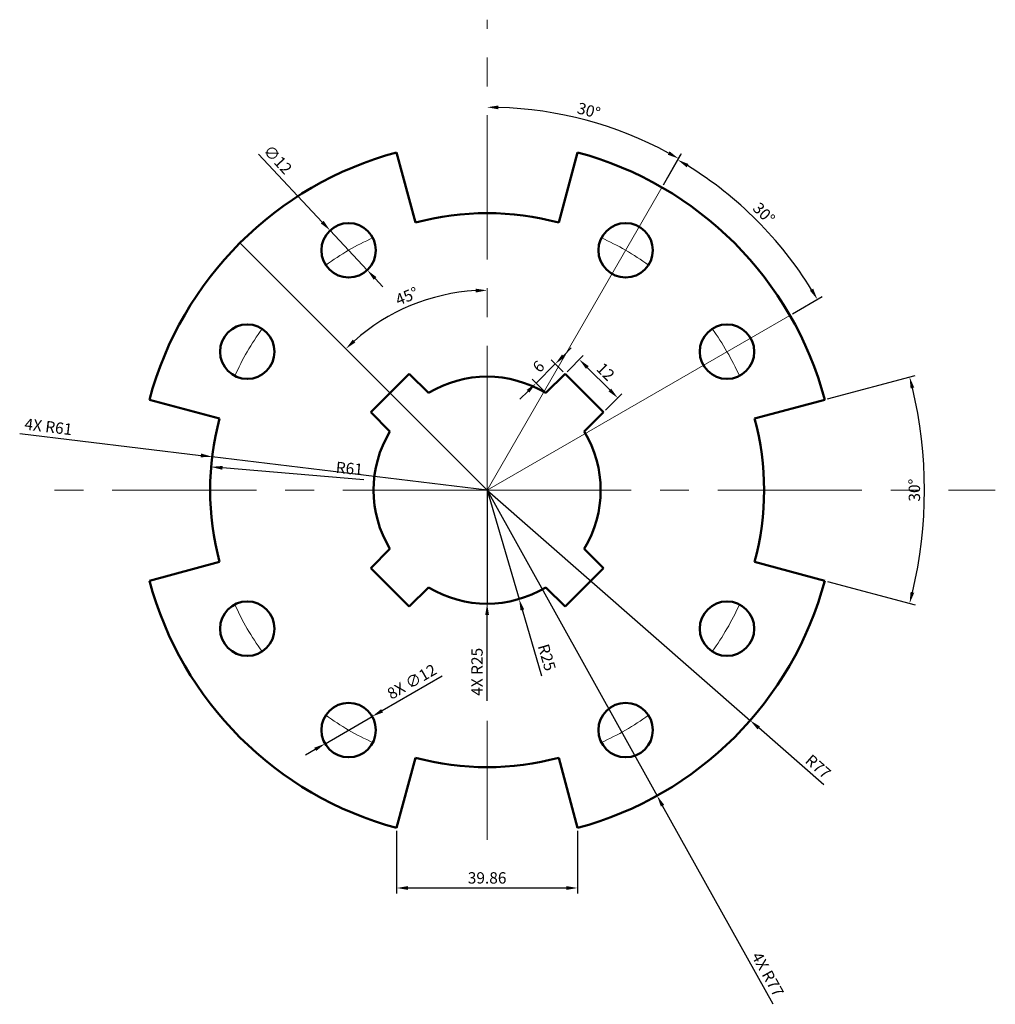
# Model space of a CAD drawing. Units: millimetres. Extents: x -38 to 176, y -46 to 171.
import ezdxf

# ---------------------------------------------------------------- set-up
doc = ezdxf.new("R2010")
doc.units = ezdxf.units.MM
doc.linetypes.add('CENTER', pattern=[50.8, 31.75, -6.35, 6.35, -6.35])
for name, color, linetype, lineweight in [('M-CNTR', 4, 'CENTER', 18), ('M-CONS', 8, 'Continuous', 13), ('M-DIMS', 2, 'Continuous', 25), ('M-OUTL', 7, 'Continuous', 50)]:
    doc.layers.add(name, color=color, linetype=linetype, lineweight=lineweight)
doc.styles.get("Standard").update_dxf_attribs({"font": 'arial.ttf'})
doc.dimstyles.new('ISO-25', dxfattribs={"dimtxt": 2.5, "dimasz": 2.5, "dimexe": 1.25, "dimexo": 0.625, "dimtad": 1, "dimtxsty": 'Standard', "dimcen": 2.5, "dimadec": 0, "dimazin": 0, "dimtfac": 1, "dimtmove": 0, "dimatfit": 3, "dimfxl": 1, "dimarcsym": 0})

# ---------------------------------------------------------------- blocks, each defined once
blk = doc.blocks.new('*U1')
for p, q in [((-6.36, 2.12), (-2.12, 6.36)), ((-2.12, 6.36), (6.36, -2.12)), ((2.12, -6.36), (6.36, -2.12))]:
    blk.add_line(p, q)
blk = doc.blocks.new('*U2')
at = {"layer": 'M-OUTL', "color": 0, "linetype": 'ByBlock', "lineweight": -2, "transparency": 16777216}
for p, rotation in [((45.29, 86.23), 90.00000000000003), ((45.29, 47.67), 180), ((83.86, 47.67), 270)]:
    blk.add_blockref('*U1', p, dxfattribs=dict(at, rotation=rotation))
blk.add_blockref('*U1', (83.86, 86.23), dxfattribs=at)
blk = doc.blocks.new('*D3')
at = {"layer": 'Defpoints', "color": 0, "transparency": 16777216}
for p in [(81.74, 92.59), (93.36, 87.25), (90.22, 84.11)]:
    blk.add_point(p, dxfattribs=at)
at = {"layer": 'M-DIMS', "color": 0, "lineweight": -2, "transparency": 16777216}
for p, q in [((82.18, 93.04), (85.76, 96.62)), ((86.64, 93.97), (91.59, 89.02)), ((90.66, 84.55), (94.24, 88.13))]:
    blk.add_line(p, q, dxfattribs=at)
at = {"layer": 'M-DIMS', "color": 0, "transparency": 16777216}
for points in [[(86.94, 94.26), (86.35, 93.67), (84.87, 95.73)], [(91.89, 89.31), (91.3, 88.72), (93.36, 87.25)]]:
    blk.add_solid(points, dxfattribs=at)
at = {"layer": 'M-DIMS', "color": 0, "transparency": 16777216, "insert": (90.45, 92.82), "char_height": 2.5, "attachment_point": 5, "rotation": 315}
blk.add_mtext('12', dxfattribs=at)
blk = doc.blocks.new('*D4')
at = {"layer": 'Defpoints', "color": 0, "transparency": 16777216}
for p in [(79.59, 94.74), (81.74, 92.59), (77.49, 88.35)]:
    blk.add_point(p, dxfattribs=at)
at = {"layer": 'M-DIMS', "color": 0, "lineweight": -2, "transparency": 16777216}
for p, q in [((81.36, 96.51), (83.12, 98.28)), ((81.29, 93.04), (78.7, 95.63)), ((75.35, 90.5), (79.59, 94.74)), ((77.05, 88.79), (74.46, 91.38)), ((73.58, 88.73), (71.81, 86.96))]:
    blk.add_line(p, q, dxfattribs=at)
at = {"layer": 'M-DIMS', "color": 0, "transparency": 16777216}
for points in [[(81.06, 96.8), (81.65, 96.21), (79.59, 94.74)], [(73.28, 89.03), (73.87, 88.44), (75.35, 90.5)]]:
    blk.add_solid(points, dxfattribs=at)
at = {"layer": 'M-DIMS', "color": 0, "transparency": 16777216, "insert": (76.12, 93.96), "char_height": 2.5, "attachment_point": 5, "rotation": 45}
blk.add_mtext('6', dxfattribs=at)
blk = doc.blocks.new('*D5')
at = {"layer": 'Defpoints', "color": 0, "transparency": 16777216}
for p in [(64.57, 170.55), (10.13, 121.39), (53.18, 109.46), (64.57, 66.95), (64.57, 66.95)]:
    blk.add_point(p, dxfattribs=at)
at = {"layer": 'M-DIMS', "color": 0, "lineweight": -2, "transparency": 16777216}
blk.add_arc((64.57, 66.95), 44.01, 93.255, 131.745, dxfattribs=at)
at = {"layer": 'M-DIMS', "color": 0, "transparency": 16777216}
for points in [[(62.06, 111.31), (62.09, 110.47), (64.57, 110.96)], [(35.56, 99.48), (34.98, 100.09), (33.45, 98.07)]]:
    blk.add_solid(points, dxfattribs=at)
at = {"layer": 'M-DIMS', "color": 0, "transparency": 16777216, "insert": (47.01, 109.36), "char_height": 2.5, "attachment_point": 5, "rotation": 22.5}
blk.add_mtext('45°', dxfattribs=at)
blk = doc.blocks.new('*D6')
at = {"layer": 'Defpoints', "color": 0, "transparency": 16777216}
for p in [(138.95, 86.88), (123.5, 82.74), (160.54, 58.55), (123.5, 51.16), (138.95, 47.02)]:
    blk.add_point(p, dxfattribs=at)
at = {"layer": 'M-DIMS', "color": 0, "lineweight": -2, "transparency": 16777216}
for p, q in [((139.55, 87.04), (158.83, 92.2)), ((139.55, 46.86), (158.83, 41.69))]:
    blk.add_line(p, q, dxfattribs=at)
blk.add_arc((64.57, 66.95), 96.33, 346.487, 13.513, dxfattribs=at)
at = {"layer": 'M-DIMS', "color": 0, "transparency": 16777216}
for points in [[(157.84, 89.35), (158.64, 89.56), (157.62, 91.88)], [(158.64, 44.34), (157.84, 44.54), (157.62, 42.02)]]:
    blk.add_solid(points, dxfattribs=at)
at = {"layer": 'M-DIMS', "color": 0, "transparency": 16777216, "insert": (159, 66.95), "char_height": 2.5, "attachment_point": 5, "rotation": 90}
blk.add_mtext('30°', dxfattribs=at)
blk = doc.blocks.new('*D7')
at = {"layer": 'Defpoints', "color": 0, "transparency": 16777216}
for p in [(64.57, 170.55), (93.41, 146.18), (103.07, 133.63), (64.57, 66.95), (64.57, 66.95)]:
    blk.add_point(p, dxfattribs=at)
at = {"layer": 'M-DIMS', "color": 0, "lineweight": -2, "transparency": 16777216}
blk.add_line((103.39, 134.17), (107.36, 141.05), dxfattribs=at)
blk.add_arc((64.57, 66.95), 84.32, 61.6989, 88.3011, dxfattribs=at)
at = {"layer": 'M-DIMS', "color": 0, "transparency": 16777216}
for points in [[(67.07, 150.81), (67.08, 151.65), (64.57, 151.27)], [(104.75, 141.55), (104.35, 140.82), (106.73, 139.97)]]:
    blk.add_solid(points, dxfattribs=at)
at = {"layer": 'M-DIMS', "color": 0, "transparency": 16777216, "insert": (86.89, 150.23), "char_height": 2.5, "attachment_point": 5, "rotation": 345}
blk.add_mtext('30°', dxfattribs=at)
blk = doc.blocks.new('*D8')
at = {"layer": 'Defpoints', "color": 0, "transparency": 16777216}
for p in [(103.07, 133.63), (128.92, 120.94), (131.26, 105.45), (64.57, 66.95), (64.57, 66.95)]:
    blk.add_point(p, dxfattribs=at)
at = {"layer": 'M-DIMS', "color": 0, "lineweight": -2, "transparency": 16777216}
for p, q in [((103.39, 134.17), (107.2, 140.77)), ((131.8, 105.76), (138.4, 109.57))]:
    blk.add_line(p, q, dxfattribs=at)
blk.add_arc((64.57, 66.95), 84, 31.7054, 58.2946, dxfattribs=at)
at = {"layer": 'M-DIMS', "color": 0, "transparency": 16777216}
for points in [[(108.51, 138.05), (108.93, 138.77), (106.57, 139.69)], [(136.39, 111.31), (135.68, 110.88), (137.32, 108.95)]]:
    blk.add_solid(points, dxfattribs=at)
at = {"layer": 'M-DIMS', "color": 0, "transparency": 16777216, "insert": (125.31, 127.69), "char_height": 2.5, "attachment_point": 5, "rotation": 315}
blk.add_mtext('30°', dxfattribs=at)
blk = doc.blocks.new('*D9')
at = {"layer": 'Defpoints', "color": 0, "transparency": 16777216}
for p in [(29.97, 124.15), (38.18, 115.4)]:
    blk.add_point(p, dxfattribs=at)
at = {"layer": 'M-DIMS', "color": 0, "lineweight": -2, "transparency": 16777216}
for p, q in [((14.22, 140.93), (28.26, 125.97)), ((38.18, 115.4), (29.97, 124.15)), ((39.89, 113.58), (41.6, 111.75))]:
    blk.add_line(p, q, dxfattribs=at)
at = {"layer": 'M-DIMS', "color": 0, "transparency": 16777216}
for points in [[(28.56, 126.26), (27.95, 125.69), (29.97, 124.15)], [(40.2, 113.86), (39.59, 113.29), (38.18, 115.4)]]:
    blk.add_solid(points, dxfattribs=at)
at = {"layer": 'M-DIMS', "color": 0, "transparency": 16777216, "insert": (18.23, 139.53), "char_height": 2.5, "attachment_point": 5, "rotation": 313.1862}
blk.add_mtext('∅12', dxfattribs=at)
blk = doc.blocks.new('*D10')
at = {"layer": 'Defpoints', "color": 0, "transparency": 16777216}
for p in [(64.57, 66.95), (122.52, 16.24)]:
    blk.add_point(p, dxfattribs=at)
at = {"layer": 'M-DIMS', "color": 0, "lineweight": -2, "transparency": 16777216}
for p, q in [((64.57, 66.95), (122.52, 16.24)), ((138.74, 2.05), (124.4, 14.59))]:
    blk.add_line(p, q, dxfattribs=at)
at = {"layer": 'M-DIMS', "color": 0, "transparency": 16777216}
blk.add_solid([(124.68, 14.91), (124.13, 14.28), (122.52, 16.24)], dxfattribs=at)
at = {"layer": 'M-DIMS', "color": 0, "transparency": 16777216, "insert": (137.26, 5.84), "char_height": 2.5, "attachment_point": 5, "rotation": 318.8112}
blk.add_mtext('R77', dxfattribs=at)
blk = doc.blocks.new('*D11')
at = {"layer": 'Defpoints', "color": 0, "transparency": 16777216}
for p in [(64.57, 66.95), (71.63, 42.96)]:
    blk.add_point(p, dxfattribs=at)
at = {"layer": 'M-DIMS', "color": 0, "lineweight": -2, "transparency": 16777216}
for p, q in [((64.57, 66.95), (71.63, 42.96)), ((76.62, 26.02), (72.34, 40.57))]:
    blk.add_line(p, q, dxfattribs=at)
at = {"layer": 'M-DIMS', "color": 0, "transparency": 16777216}
blk.add_solid([(72.74, 40.68), (71.94, 40.45), (71.63, 42.96)], dxfattribs=at)
at = {"layer": 'M-DIMS', "color": 0, "transparency": 16777216, "insert": (77.42, 30.03), "char_height": 2.5, "attachment_point": 5, "rotation": 286.3939}
blk.add_mtext('R25', dxfattribs=at)
blk = doc.blocks.new('*D12')
at = {"layer": 'Defpoints', "color": 0, "transparency": 16777216}
for p in [(3.79, 72.07), (64.57, 66.95)]:
    blk.add_point(p, dxfattribs=at)
at = {"layer": 'M-DIMS', "color": 0, "lineweight": -2, "transparency": 16777216}
blk.add_line((37.41, 69.24), (6.28, 71.86), dxfattribs=at)
at = {"layer": 'M-DIMS', "color": 0, "transparency": 16777216}
blk.add_solid([(6.32, 72.28), (6.25, 71.45), (3.79, 72.07)], dxfattribs=at)
at = {"layer": 'M-DIMS', "color": 0, "transparency": 16777216, "insert": (34.21, 71.42), "char_height": 2.5, "attachment_point": 5, "rotation": 355.1793}
blk.add_mtext('R61', dxfattribs=at)
blk = doc.blocks.new('BOLT-HOLE-D12')
blk.add_circle((6, 6), 6)
blk = doc.blocks.new('*D14')
at = {"layer": 'Defpoints', "color": 0, "transparency": 16777216}
for p in [(44.65, -7.43), (84.5, -7.43), (84.5, -20.65)]:
    blk.add_point(p, dxfattribs=at)
at = {"layer": 'M-DIMS', "color": 0, "lineweight": -2, "transparency": 16777216}
for p, q in [((44.65, -8.05), (44.65, -21.9)), ((84.5, -8.05), (84.5, -21.9)), ((47.15, -20.65), (82, -20.65))]:
    blk.add_line(p, q, dxfattribs=at)
at = {"layer": 'M-DIMS', "color": 0, "transparency": 16777216}
for points in [[(47.15, -20.24), (47.15, -21.07), (44.65, -20.65)], [(82, -20.24), (82, -21.07), (84.5, -20.65)]]:
    blk.add_solid(points, dxfattribs=at)
at = {"layer": 'M-DIMS', "color": 0, "transparency": 16777216, "insert": (64.57, -18.75), "char_height": 2.5, "attachment_point": 5}
blk.add_mtext('39.86', dxfattribs=at)
blk = doc.blocks.new('*D15')
at = {"layer": 'Defpoints', "color": 0, "transparency": 16777216}
for p in [(64.57, 66.95), (102, -0.34)]:
    blk.add_point(p, dxfattribs=at)
at = {"layer": 'M-DIMS', "color": 0, "lineweight": -2, "transparency": 16777216}
for p, q in [((64.57, 66.95), (102, -0.34)), ((127.55, -46.27), (103.22, -2.53))]:
    blk.add_line(p, q, dxfattribs=at)
at = {"layer": 'M-DIMS', "color": 0, "transparency": 16777216}
blk.add_solid([(103.58, -2.33), (102.85, -2.73), (102, -0.34)], dxfattribs=at)
at = {"layer": 'M-DIMS', "color": 0, "transparency": 16777216, "insert": (126.1, -39.81), "char_height": 2.5, "attachment_point": 5, "rotation": 299.0841}
blk.add_mtext('4X R77', dxfattribs=at)
blk = doc.blocks.new('*D16')
at = {"layer": 'Defpoints', "color": 0, "transparency": 16777216}
for p in [(4.02, 74.3), (64.57, 66.95)]:
    blk.add_point(p, dxfattribs=at)
at = {"layer": 'M-DIMS', "color": 0, "lineweight": -2, "transparency": 16777216}
for p, q in [((-38.38, 79.45), (1.54, 74.61)), ((64.57, 66.95), (4.02, 74.3))]:
    blk.add_line(p, q, dxfattribs=at)
at = {"layer": 'M-DIMS', "color": 0, "transparency": 16777216}
blk.add_solid([(1.59, 75.02), (1.49, 74.19), (4.02, 74.3)], dxfattribs=at)
at = {"layer": 'M-DIMS', "color": 0, "transparency": 16777216, "insert": (-32.08, 80.6), "char_height": 2.5, "attachment_point": 5, "rotation": 353.0739}
blk.add_mtext('4X R61', dxfattribs=at)
blk = doc.blocks.new('*D17')
at = {"layer": 'Defpoints', "color": 0, "transparency": 16777216}
for p in [(64.57, 66.95), (64.57, 41.95)]:
    blk.add_point(p, dxfattribs=at)
at = {"layer": 'M-DIMS', "color": 0, "lineweight": -2, "transparency": 16777216}
for p, q in [((64.57, 66.95), (64.57, 41.95)), ((64.57, 20.59), (64.57, 39.45))]:
    blk.add_line(p, q, dxfattribs=at)
at = {"layer": 'M-DIMS', "color": 0, "transparency": 16777216}
blk.add_solid([(64.16, 39.45), (64.99, 39.45), (64.57, 41.95)], dxfattribs=at)
at = {"layer": 'M-DIMS', "color": 0, "transparency": 16777216, "insert": (62.67, 26.95), "char_height": 2.5, "attachment_point": 5, "rotation": 89.9993}
blk.add_mtext('4X R25', dxfattribs=at)
blk = doc.blocks.new('*D18')
at = {"layer": 'Defpoints', "color": 0, "transparency": 16777216}
for p in [(39.27, 17.12), (28.88, 11.12)]:
    blk.add_point(p, dxfattribs=at)
at = {"layer": 'M-DIMS', "color": 0, "lineweight": -2, "transparency": 16777216}
for p, q in [((54.67, 25.99), (41.44, 18.36)), ((28.88, 11.12), (39.27, 17.12)), ((26.71, 9.88), (24.54, 8.63))]:
    blk.add_line(p, q, dxfattribs=at)
at = {"layer": 'M-DIMS', "color": 0, "transparency": 16777216}
for points in [[(41.23, 18.73), (41.65, 18), (39.27, 17.12)], [(26.5, 10.24), (26.92, 9.52), (28.88, 11.12)]]:
    blk.add_solid(points, dxfattribs=at)
at = {"layer": 'M-DIMS', "color": 0, "transparency": 16777216, "insert": (48.15, 24.51), "char_height": 2.5, "attachment_point": 5, "rotation": 29.9531}
blk.add_mtext('8X ∅12', dxfattribs=at)

msp = doc.modelspace()

# ---------------------------------------------------------------- linework, layer by layer
at = {"layer": 'M-CNTR'}
for q in [(64.574, 170.55), (-32.975, 66.948), (176.499, 66.948), (64.574, -10.052)]:
    msp.add_line((64.574, 66.948), q, dxfattribs=at)
for start, end in [(114.36208, 125.63792), (54.36208, 65.63792), (144.36208, 155.63792), (24.36208, 35.63792), (204.36208, 215.63792), (324.36208, 335.63792), (234.36208, 245.63792), (294.36208, 305.63792)]:
    msp.add_arc((64.574, 66.948), 61, start, end, dxfattribs=at)
at = {"layer": 'M-CONS'}
for q in [(103.074, 133.632), (10.127, 121.395), (131.258, 105.448)]:
    msp.add_line((64.574, 66.948), q, dxfattribs=at)
at = {"layer": 'M-OUTL'}
for p, q in [((48.786, 125.869), (44.645, 141.324)), ((80.362, 125.869), (84.503, 141.324)), ((5.653, 82.736), (-9.802, 86.877)), ((123.496, 82.736), (138.951, 86.877)), ((5.653, 51.16), (-9.802, 47.019)), ((123.496, 51.16), (138.951, 47.019)), ((48.786, 8.026), (44.645, -7.429)), ((80.362, 8.026), (84.503, -7.429))]:
    msp.add_line(p, q, dxfattribs=at)
for radius, start, end in [(77, 105, 165), (77, 15, 75), (61, 75, 105), (25, 58.88654, 121.11346), (61, 165, 195), (61, 345, 15), (25, 148.88654, 211.11346), (25, 328.88654, 31.11346), (77, 195, 255), (25, 238.88654, 301.11346), (77, 285, 345), (61, 255, 285)]:
    msp.add_arc((64.574, 66.948), radius, start, end, dxfattribs=at)

# ---------------------------------------------------------------- block references
for name, p in [('BOLT-HOLE-D12', (28.074, 113.775)), ('BOLT-HOLE-D12', (89.074, 113.775)), ('BOLT-HOLE-D12', (5.746, 91.447)), ('BOLT-HOLE-D12', (111.402, 91.447)), ('*U2', (0, 0)), ('BOLT-HOLE-D12', (5.746, 30.447)), ('BOLT-HOLE-D12', (111.402, 30.447)), ('BOLT-HOLE-D12', (28.074, 8.12)), ('BOLT-HOLE-D12', (89.074, 8.12))]:
    msp.add_blockref(name, p, dxfattribs=at)

# ---------------------------------------------------------------- dimensions: what is measured, and where the dimension line sits
at = {"layer": 'M-DIMS'}
for base, line1, line2, picture, middle in [((53.183, 109.46), ((64.574, 66.948), (64.574, 170.55)), ((64.574, 66.948), (10.127, 121.395)), '*D5', (47.006, 109.362)), ((93.413, 146.181), ((64.574, 66.948), (64.574, 170.55)), ((64.574, 66.948), (103.074, 133.632)), '*D7', (86.89, 150.23)), ((128.92, 120.94), ((64.574, 66.948), (103.074, 133.632)), ((64.574, 66.948), (131.258, 105.448)), '*D8', (125.314, 127.688)), ((160.539, 58.552), ((123.496, 82.736), (138.951, 86.877)), ((123.496, 51.16), (138.951, 47.019)), '*D6', (159.004, 66.948))]:
    dim = msp.add_angular_dim_2l(base=base, line1=line1, line2=line2, dimstyle='ISO-25', override={"dimclrd": 0, "dimclre": 0, "dimclrt": 0}, dxfattribs=at)
    dim.commit()
    dim.dimension.update_dxf_attribs({"geometry": picture, "text_midpoint": middle})
dim = msp.add_diameter_dim_2p(p1=(38.181, 115.4), p2=(29.968, 124.15), dimstyle='ISO-25', override={"dimclrd": 0, "dimclre": 0, "dimclrt": 0}, dxfattribs=at)
dim.commit()
dim.dimension.update_dxf_attribs({"geometry": '*D9', "text_midpoint": (16.797, 138.183), "dimtype": 163})
for p1, p2, distance, picture, middle in [((77.493, 88.351), (81.735, 92.594), 3.037, '*D4', (76.122, 93.965)), ((81.735, 92.594), (90.221, 84.109), 4.44, '*D3', (90.447, 92.82))]:
    dim = msp.add_aligned_dim(p1=p1, p2=p2, distance=distance, dimstyle='ISO-25', override={"dimclrd": 0, "dimclre": 0, "dimclrt": 0}, dxfattribs=at)
    dim.commit()
    dim.dimension.update_dxf_attribs({"geometry": picture, "text_midpoint": middle})
for mpoint, picture, middle in [((4.019, 74.304), '*D16', (-32.313, 78.717)), ((64.574, 41.948), '*D17', (64.574, 26.948)), ((102.003, -0.343), '*D15', (124.461, -40.718))]:
    dim = msp.add_radius_dim(center=(64.574, 66.948), mpoint=mpoint, text='4X <>', dimstyle='ISO-25', override={"dimdec": 0, "dimlfac": 1, "dimrnd": 0, "dimzin": 0, "dimdsep": 46, "dimlunit": 2}, dxfattribs=at)
    dim.commit()
    dim.dimension.update_dxf_attribs({"geometry": picture, "text_midpoint": middle, "dimtype": 164})
for mpoint, picture, middle in [((3.79, 72.074), '*D12', (34.05, 69.522)), ((122.52, 16.24), '*D10', (136.022, 4.425)), ((71.63, 42.964), '*D11', (75.595, 29.489))]:
    dim = msp.add_radius_dim(center=(64.574, 66.948), mpoint=mpoint, dimstyle='ISO-25', override={"dimclrd": 0, "dimclre": 0, "dimclrt": 0}, dxfattribs=at)
    dim.commit()
    dim.dimension.update_dxf_attribs({"geometry": picture, "text_midpoint": middle, "dimtype": 164})
dim = msp.add_diameter_dim_2p(p1=(28.876, 11.124), p2=(39.273, 17.116), text='8X <>', dimstyle='ISO-25', override={"dimdec": 0, "dimlfac": 1, "dimrnd": 0, "dimzin": 0, "dimdsep": 46, "dimlunit": 2}, dxfattribs=at)
dim.commit()
dim.dimension.update_dxf_attribs({"geometry": '*D18', "text_midpoint": (49.136, 22.8)})
dim = msp.add_linear_dim(base=(84.503, -20.652), p1=(44.645, -7.429), p2=(84.503, -7.429), dimstyle='ISO-25', override={"dimdec": 2, "dimlfac": 1, "dimrnd": 0, "dimzin": 0, "dimdsep": 46, "dimlunit": 2}, dxfattribs=at)
dim.commit()
dim.dimension.update_dxf_attribs({"geometry": '*D14', "text_midpoint": (64.574, -18.75)})

doc.saveas('drawing.dxf')
